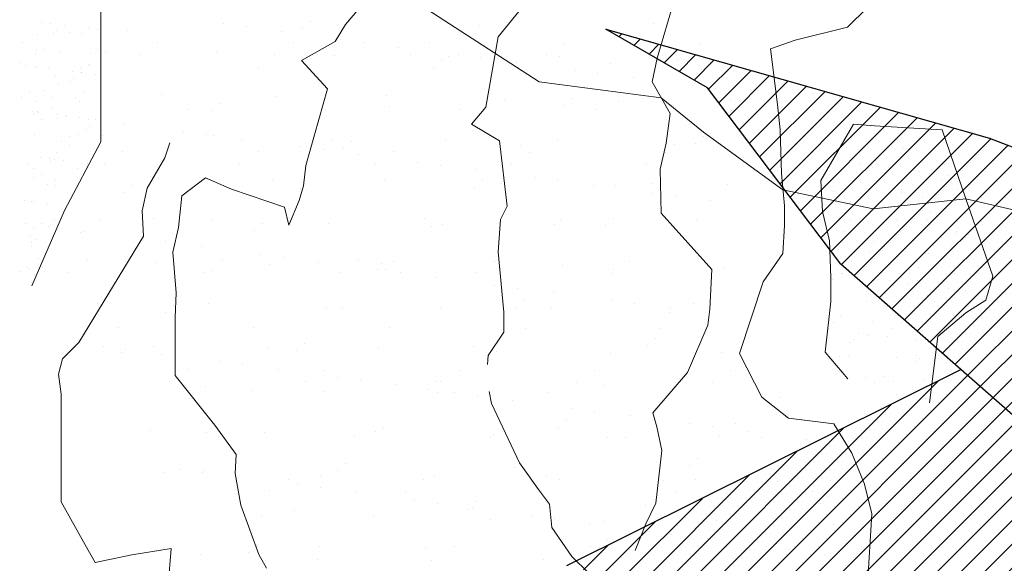
# Model space of a CAD drawing. Units: inches. Extents: x 1986 to 21484, y -1816 to 2016.
# Tile 17 of 85: x 2148.647 to 2157.681, y 1882.437 to 1887.425. Entities that reach past the tile are written whole.
import ezdxf

# ---------------------------------------------------------------- set-up
doc = ezdxf.new("R2010")
doc.units = ezdxf.units.IN
doc.layers.add('L-PLNT', color=84, linetype='Continuous', lineweight=13)
doc.layers.add('vfolhas', color=114, linetype='Continuous', lineweight=5)
doc.layers.add('vfolhas2', color=102, linetype='Continuous')

# ---------------------------------------------------------------- blocks, each defined once
blk = doc.blocks.new('arbusto_PB_verde_grande')
at = {"layer": 'vfolhas'}
h = blk.add_hatch(dxfattribs=at)
h.set_pattern_fill('ANSI31', color=256, scale=0.05, style=0)
h.set_pattern_definition([(45, (-2446.5133113, 50.986076), (-0.004419417382, 0.004419417382), [])])
h.paths.add_polyline_path([(-0.57219, 0.06233), (-0.7153, 0.10298), (-0.67736, 0.08107), (-0.62769, 0.01536), (-0.56347, -0.04095), (-0.26461, -0.0834), (-0.14874, -0.06595), (-0.10151, -0.05877), (-0.20418, -0.0472), (-0.40279, -0.00339)])
h.paths.add_polyline_path([(-0.56347, -0.04095), (-0.58279, -0.02401), (-0.72992, -0.09726), (-0.4334, -0.1679), (-0.41452, -0.15048), (-0.31518, -0.09101), (-0.26461, -0.0834)])
h.paths.add_polyline_path([(-0.2769, -0.47267), (-0.27429, -0.44776), (-0.16328, -0.25376), (0.02625, -0.03934), (-0.21007, -0.20995), (-0.2672, -0.24466), (-0.36485, -0.35697), (-0.42907, -0.46341), (-0.47586, -0.60425), (-0.37946, -0.57603)])
at = {"layer": 'vfolhas2'}
for p, q in [((-0.67736, 0.08107), (-0.7153, 0.10298)), ((-0.7153, 0.10298), (-0.57219, 0.06233)), ((-0.62769, 0.01536), (-0.67736, 0.08107)), ((-0.57219, 0.06233), (-0.40279, -0.00339)), ((-0.56347, -0.04095), (-0.62769, 0.01536)), ((-0.58279, -0.02401), (-0.72992, -0.09726))]:
    blk.add_line(p, q, dxfattribs=at)
blk = doc.blocks.new('PLANT-SHRUB')
for p, q in [((2149.3904, 1887.9573), (2149.3904, 1887.2965)), ((2151.874, 1887.8531), (2153.4137, 1886.8553)), ((2154.6784, 1887.6913), (2154.4964, 1887.0728)), ((2153.0377, 1887.2662), (2153.2939, 1887.5837)), ((2151.636, 1887.381), (2151.7601, 1887.5256)), ((2156.2426, 1887.3561), (2156.4241, 1887.5374)), ((2151.3125, 1887.4075), (2151.3125, 1887.4075)), ((2148.847, 1887.3985), (2148.847, 1887.3985)), ((2148.9303, 1887.3876), (2148.9303, 1887.3876)), ((2148.9856, 1887.3277), (2148.9856, 1887.3277)), ((2149.0602, 1887.3705), (2149.0602, 1887.3705)), ((2149.2774, 1887.3419), (2149.2774, 1887.3419)), ((2149.3606, 1887.3309), (2149.3606, 1887.3309)), ((2149.6396, 1887.3262), (2149.6396, 1887.3262)), ((2150.5172, 1887.3856), (2150.5172, 1887.3856)), ((2150.7253, 1887.3582), (2150.7253, 1887.3582)), ((2151.0502, 1887.3155), (2151.0502, 1887.3155)), ((2151.2389, 1887.34), (2151.2389, 1887.34)), ((2151.543, 1887.226), (2151.636, 1887.381)), ((2152.8617, 1887.3753), (2152.8617, 1887.3753)), ((2154.461, 1887.389), (2154.461, 1887.389)), ((2155.7616, 1887.2382), (2156.2426, 1887.3561)), ((2156.2426, 1887.3561), (2156.2426, 1887.3561)), ((2148.8099, 1887.2924), (2148.8099, 1887.2924)), ((2148.9562, 1887.3007), (2148.9562, 1887.3007)), ((2149.1052, 1887.3099), (2149.1052, 1887.3099)), ((2149.2189, 1887.2943), (2149.2189, 1887.2943)), ((2149.3904, 1887.2965), (2149.3904, 1886.876)), ((2151.2327, 1887.0503), (2151.543, 1887.226)), ((2151.5931, 1887.244), (2151.5931, 1887.244)), ((2152.9249, 1886.6211), (2153.0377, 1887.2662)), ((2155.5347, 1887.1566), (2155.7616, 1887.2382)), ((2148.6687, 1887.2197), (2148.6687, 1887.2197)), ((2148.797, 1887.1549), (2148.797, 1887.1549)), ((2148.8625, 1887.1553), (2148.8625, 1887.1553)), ((2149.016, 1887.1342), (2149.016, 1887.1342)), ((2149.3603, 1887.1543), (2149.3603, 1887.1543)), ((2149.4326, 1887.1303), (2149.4326, 1887.1303)), ((2149.9133, 1887.2174), (2149.9133, 1887.2174)), ((2150.455, 1887.1352), (2150.455, 1887.1352)), ((2151.1579, 1887.2152), (2151.1579, 1887.2152)), ((2151.8011, 1887.2166), (2151.8011, 1887.2166)), ((2152.126, 1887.1738), (2152.126, 1887.1738)), ((2152.4026, 1887.2129), (2152.4026, 1887.2129)), ((2153.6472, 1887.2106), (2153.6472, 1887.2106)), ((2154.8918, 1887.2084), (2154.8918, 1887.2084)), ((2155.5986, 1886.6458), (2155.5347, 1887.1566)), ((2148.7951, 1887.1123), (2148.7951, 1887.1123)), ((2149.2929, 1887.1114), (2149.2929, 1887.1114)), ((2149.7448, 1887.11), (2149.7448, 1887.11)), ((2150.9894, 1887.1078), (2150.9894, 1887.1078)), ((2151.4706, 1886.7919), (2151.2327, 1887.0503)), ((2151.5345, 1887.0963), (2151.5345, 1887.0963)), ((2152.234, 1887.1055), (2152.234, 1887.1055)), ((2152.514, 1887.0567), (2152.514, 1887.0567)), ((2152.5806, 1887.083), (2152.5806, 1887.083)), ((2152.6689, 1887.1023), (2152.6689, 1887.1023)), ((2152.8769, 1887.075), (2152.8769, 1887.075)), ((2153.4787, 1887.1033), (2153.4787, 1887.1033)), ((2153.603, 1887.0879), (2153.603, 1887.0879)), ((2154.4964, 1887.0728), (2154.4509, 1886.8545)), ((2154.6825, 1887.049), (2154.6825, 1887.049)), ((2154.7233, 1887.101), (2154.7233, 1887.101)), ((2148.6579, 1887.0275), (2148.6579, 1887.0275)), ((2148.6997, 1887.004), (2148.6997, 1887.004)), ((2148.7829, 1886.9931), (2148.7829, 1886.9931)), ((2148.7999, 1886.9843), (2148.7999, 1886.9843)), ((2148.9128, 1886.976), (2148.9128, 1886.976)), ((2149.2088, 1886.9863), (2149.2088, 1886.9863)), ((2149.2776, 1887.0146), (2149.2776, 1887.0146)), ((2149.2919, 1887.0076), (2149.2919, 1887.0076)), ((2150.8411, 1886.9754), (2150.8411, 1886.9754)), ((2152.4403, 1886.9892), (2152.4403, 1886.9892)), ((2153.2019, 1887.0322), (2153.2019, 1887.0322)), ((2153.7447, 1886.9607), (2153.7447, 1886.9607)), ((2154.0632, 1887.0245), (2154.0632, 1887.0245)), ((2148.9761, 1886.9095), (2148.9761, 1886.9095)), ((2149.1091, 1886.8601), (2149.1091, 1886.8601)), ((2149.13, 1886.9474), (2149.13, 1886.9474)), ((2149.1385, 1886.8871), (2149.1385, 1886.8871)), ((2149.2132, 1886.9364), (2149.2132, 1886.9364)), ((2149.2182, 1886.9401), (2149.2182, 1886.9401)), ((2149.3432, 1886.9193), (2149.3432, 1886.9193)), ((2149.3904, 1886.876), (2149.3904, 1886.3054)), ((2153.9528, 1886.9333), (2153.9528, 1886.9333)), ((2154.2777, 1886.8905), (2154.2777, 1886.8905)), ((2148.8684, 1886.7739), (2148.8684, 1886.7739)), ((2149.006, 1886.8262), (2149.006, 1886.8262)), ((2151.2728, 1886.0864), (2151.4706, 1886.7919)), ((2153.4137, 1886.8553), (2154.5328, 1886.7089)), ((2154.4509, 1886.8545), (2154.6147, 1886.5634)), ((2154.8205, 1886.8191), (2154.8205, 1886.8191)), ((2155.0286, 1886.7917), (2155.0286, 1886.7917)), ((2148.666, 1886.712), (2148.666, 1886.712)), ((2148.7334, 1886.7549), (2148.7334, 1886.7549)), ((2148.9499, 1886.7143), (2148.9499, 1886.7143)), ((2149.1638, 1886.7111), (2149.1638, 1886.7111)), ((2149.1988, 1886.6782), (2149.1988, 1886.6782)), ((2149.2312, 1886.754), (2149.2312, 1886.754)), ((2149.9479, 1886.735), (2149.9479, 1886.735)), ((2150.994, 1886.7216), (2150.994, 1886.7216)), ((2152.0164, 1886.7265), (2152.0164, 1886.7265)), ((2153.0959, 1886.6876), (2153.0959, 1886.6876)), ((2153.7155, 1886.7059), (2153.7155, 1886.7059)), ((2154.5328, 1886.7089), (2154.9211, 1886.3936)), ((2155.1645, 1886.6792), (2155.1645, 1886.6792)), ((2155.3535, 1886.7489), (2155.3535, 1886.7489)), ((2148.7898, 1886.6763), (2148.7898, 1886.6763)), ((2148.9526, 1886.6054), (2148.9526, 1886.6054)), ((2150.1973, 1886.6031), (2150.1973, 1886.6031)), ((2150.4197, 1886.5893), (2150.4197, 1886.5893)), ((2150.4934, 1886.6568), (2150.4934, 1886.6568)), ((2151.4419, 1886.6009), (2151.4419, 1886.6009)), ((2152.0425, 1886.6247), (2152.0425, 1886.6247)), ((2152.6865, 1886.5986), (2152.6865, 1886.5986)), ((2152.7917, 1886.4675), (2152.9249, 1886.6211)), ((2153.6418, 1886.6384), (2153.6418, 1886.6384)), ((2153.9312, 1886.5963), (2153.9312, 1886.5963)), ((2154.1421, 1886.6743), (2154.1421, 1886.6743)), ((2155.1758, 1886.5941), (2155.1758, 1886.5941)), ((2155.2646, 1886.6737), (2155.2646, 1886.6737)), ((2155.6244, 1886.4136), (2155.5986, 1886.6458)), ((2148.7654, 1886.5814), (2148.7654, 1886.5814)), ((2148.7814, 1886.5599), (2148.7814, 1886.5599)), ((2148.8109, 1886.5869), (2148.8109, 1886.5869)), ((2148.8204, 1886.5756), (2148.8204, 1886.5756)), ((2148.847, 1886.5092), (2148.847, 1886.5092)), ((2148.9826, 1886.5529), (2148.9826, 1886.5529)), ((2148.9959, 1886.5181), (2148.9959, 1886.5181)), ((2149.0658, 1886.5419), (2149.0658, 1886.5419)), ((2149.0729, 1886.541), (2149.0729, 1886.541)), ((2149.1958, 1886.5248), (2149.1958, 1886.5248)), ((2149.281, 1886.5136), (2149.281, 1886.5136)), ((2149.3448, 1886.5083), (2149.3448, 1886.5083)), ((2154.6147, 1886.5634), (2154.5783, 1886.2905)), ((2149.262, 1886.4196), (2149.262, 1886.4196)), ((2149.2914, 1886.4466), (2149.2914, 1886.4466)), ((2149.6059, 1886.4708), (2149.6059, 1886.4708)), ((2152.7917, 1886.4675), (2152.7917, 1886.4675)), ((2153.0479, 1886.3139), (2152.7917, 1886.4675)), ((2155.6373, 1886.0136), (2155.6244, 1886.4136)), ((2156.2958, 1886.4652), (2155.9988, 1885.9491)), ((2156.4895, 1886.4523), (2156.2958, 1886.4652)), ((2157.1093, 1886.4136), (2156.4895, 1886.4523)), ((2157.3288, 1885.7813), (2157.1093, 1886.4136)), ((2148.7797, 1886.3682), (2148.7797, 1886.3682)), ((2149.1021, 1886.3537), (2149.1021, 1886.3537)), ((2149.1887, 1886.3702), (2149.1887, 1886.3702)), ((2149.4074, 1886.3602), (2149.4074, 1886.3602)), ((2150.1488, 1886.3993), (2150.1488, 1886.3993)), ((2150.3568, 1886.3719), (2150.3568, 1886.3719)), ((2150.4298, 1886.3651), (2150.4298, 1886.3651)), ((2150.6817, 1886.3292), (2150.6817, 1886.3292)), ((2151.5093, 1886.3263), (2151.5093, 1886.3263)), ((2153.5779, 1886.3178), (2153.5779, 1886.3178)), ((2154.9169, 1886.3551), (2154.9169, 1886.3551)), ((2154.9211, 1886.3936), (2155.6502, 1885.8652)), ((2156.2786, 1886.3449), (2156.2786, 1886.3449)), ((2156.7369, 1886.3459), (2156.7369, 1886.3459)), ((2156.9009, 1886.3437), (2156.9009, 1886.3437)), ((2149.0347, 1886.3107), (2149.0347, 1886.3107)), ((2149.3904, 1886.3054), (2149.0597, 1885.6747)), ((2149.1029, 1886.2738), (2149.1029, 1886.2738)), ((2150.0259, 1886.2961), (2149.9795, 1886.157)), ((2151.2246, 1886.2577), (2151.2246, 1886.2577)), ((2151.4326, 1886.2303), (2151.4326, 1886.2303)), ((2151.6212, 1886.2385), (2151.6212, 1886.2385)), ((2151.6948, 1886.3061), (2151.6948, 1886.3061)), ((2152.5555, 1886.3129), (2152.5555, 1886.3129)), ((2153.1193, 1885.7143), (2153.0479, 1886.3139)), ((2153.244, 1886.2739), (2153.244, 1886.2739)), ((2154.5783, 1886.2905), (2154.5237, 1886.054)), ((2154.6573, 1886.2789), (2154.6573, 1886.2789)), ((2154.8433, 1886.2876), (2154.8433, 1886.2876)), ((2156.2313, 1886.2553), (2156.2313, 1886.2553)), ((2156.7001, 1886.3122), (2156.7001, 1886.3122)), ((2156.7544, 1886.2486), (2156.7544, 1886.2486)), ((2148.8352, 1886.1583), (2148.8352, 1886.1583)), ((2148.9184, 1886.1474), (2148.9184, 1886.1474)), ((2148.9638, 1886.1463), (2148.9638, 1886.1463)), ((2148.9858, 1886.2101), (2148.9858, 1886.2101)), ((2149.5905, 1886.2166), (2149.5905, 1886.2166)), ((2149.9795, 1886.157), (2149.8169, 1885.8786)), ((2150.0219, 1886.2248), (2150.0219, 1886.2248)), ((2150.8351, 1886.2143), (2150.8351, 1886.2143)), ((2151.7575, 1886.1875), (2151.7575, 1886.1875)), ((2152.0798, 1886.2121), (2152.0798, 1886.2121)), ((2153.3244, 1886.2098), (2153.3244, 1886.2098)), ((2154.569, 1886.2075), (2154.569, 1886.2075)), ((2156.5975, 1886.1505), (2156.5975, 1886.1505)), ((2148.7179, 1886.1089), (2148.7179, 1886.1089)), ((2148.7697, 1886.0602), (2148.7697, 1886.0602)), ((2148.9343, 1886.1193), (2148.9343, 1886.1193)), ((2149.0484, 1886.1303), (2149.0484, 1886.1303)), ((2149.1786, 1886.0622), (2149.1786, 1886.0622)), ((2149.2157, 1886.108), (2149.2157, 1886.108)), ((2149.2655, 1886.1017), (2149.2655, 1886.1017)), ((2149.422, 1886.1092), (2149.422, 1886.1092)), ((2150.6666, 1886.107), (2150.6666, 1886.107)), ((2151.2521, 1885.9004), (2151.2728, 1886.0864)), ((2151.9112, 1886.1047), (2151.9112, 1886.1047)), ((2152.3004, 1886.1161), (2152.3004, 1886.1161)), ((2152.5084, 1886.0887), (2152.5084, 1886.0887)), ((2152.8334, 1886.0459), (2152.8334, 1886.0459)), ((2153.1559, 1886.1024), (2153.1559, 1886.1024)), ((2154.4005, 1886.1002), (2154.4005, 1886.1002)), ((2154.5237, 1886.054), (2154.5332, 1885.65)), ((2156.354, 1886.0998), (2156.354, 1886.0998)), ((2156.4581, 1886.0861), (2156.4581, 1886.0861)), ((2156.4723, 1886.0703), (2156.4723, 1886.0703)), ((2156.5012, 1886.1299), (2156.5012, 1886.1299)), ((2156.5132, 1886.0968), (2156.5132, 1886.0968)), ((2156.6205, 1886.0647), (2156.6205, 1886.0647)), ((2157.0121, 1886.0509), (2157.0121, 1886.0509)), ((2157.1356, 1886.0957), (2157.1356, 1886.0957)), ((2148.7752, 1885.9735), (2148.7752, 1885.9735)), ((2148.8432, 1886.0038), (2148.8432, 1886.0038)), ((2149.9227, 1885.9649), (2149.9227, 1885.9649)), ((2150.1352, 1885.8074), (2150.3524, 1885.9727)), ((2150.3524, 1885.9727), (2150.5903, 1885.8694)), ((2150.3524, 1885.9727), (2150.3524, 1885.9727)), ((2151.9913, 1885.9564), (2151.9913, 1885.9564)), ((2152.8963, 1885.9553), (2152.8963, 1885.9553)), ((2153.3762, 1885.9744), (2153.3762, 1885.9744)), ((2155.6631, 1885.7168), (2155.6373, 1886.0136)), ((2156.3274, 1885.9706), (2156.3274, 1885.9706)), ((2156.892, 1886.029), (2156.892, 1886.029)), ((2156.996, 1886.0153), (2156.996, 1886.0153)), ((2157.1584, 1885.9939), (2157.1584, 1885.9939)), ((2148.9056, 1885.9104), (2148.9056, 1885.9104)), ((2148.973, 1885.9534), (2148.973, 1885.9534)), ((2148.9758, 1885.9021), (2148.9758, 1885.9021)), ((2149.6742, 1885.9062), (2149.6742, 1885.9062)), ((2149.8169, 1885.8786), (2149.7705, 1885.6698)), ((2150.5903, 1885.8694), (2151.0763, 1885.7041)), ((2150.9689, 1885.9515), (2150.9689, 1885.9515)), ((2151.2108, 1885.7661), (2151.2521, 1885.9004)), ((2151.2234, 1885.874), (2151.2234, 1885.874)), ((2152.8226, 1885.8878), (2152.8226, 1885.8878)), ((2153.0707, 1885.9175), (2153.0707, 1885.9175)), ((2153.5843, 1885.947), (2153.5843, 1885.947)), ((2153.9092, 1885.9043), (2153.9092, 1885.9043)), ((2154.1169, 1885.9042), (2154.1169, 1885.9042)), ((2154.4455, 1885.9231), (2154.4455, 1885.9231)), ((2155.1393, 1885.9091), (2155.1393, 1885.9091)), ((2155.6502, 1885.8652), (2156.4772, 1885.6891)), ((2155.9988, 1885.9491), (2156.0118, 1885.6652)), ((2156.2188, 1885.8702), (2156.2188, 1885.8702)), ((2156.2905, 1885.9368), (2156.2905, 1885.9368)), ((2157.1019, 1885.9545), (2157.1019, 1885.9545)), ((2157.253, 1885.866), (2157.253, 1885.866)), ((2149.6005, 1885.8387), (2149.6005, 1885.8387)), ((2150.1042, 1885.518), (2150.1352, 1885.8074)), ((2150.1352, 1885.8074), (2150.1352, 1885.8074)), ((2154.452, 1885.8328), (2154.452, 1885.8328)), ((2154.6601, 1885.8054), (2154.6601, 1885.8054)), ((2156.1172, 1885.8445), (2156.1172, 1885.8445)), ((2156.4772, 1885.6891), (2157.3288, 1885.7813)), ((2156.7395, 1885.8433), (2156.7395, 1885.8433)), ((2156.7418, 1885.8635), (2156.7418, 1885.8635)), ((2156.9281, 1885.7952), (2156.9281, 1885.7952)), ((2157.3288, 1885.7813), (2158.2522, 1885.5676)), ((2157.5742, 1885.0717), (2157.3288, 1885.7813)), ((2148.6878, 1885.7638), (2148.6878, 1885.7638)), ((2148.7596, 1885.7522), (2148.7596, 1885.7522)), ((2148.771, 1885.7529), (2148.771, 1885.7529)), ((2148.901, 1885.7357), (2148.901, 1885.7357)), ((2151.0763, 1885.7041), (2151.1177, 1885.5387)), ((2151.1177, 1885.5387), (2151.2108, 1885.7661)), ((2151.2108, 1885.7661), (2151.2108, 1885.7661)), ((2153.0578, 1885.5914), (2153.1193, 1885.7143)), ((2153.1193, 1885.7143), (2153.1193, 1885.7143)), ((2154.985, 1885.7626), (2154.985, 1885.7626)), ((2155.6631, 1885.5362), (2155.6631, 1885.7168)), ((2156.0916, 1885.7546), (2156.0916, 1885.7546)), ((2156.4597, 1885.6853), (2156.4597, 1885.6853)), ((2156.8913, 1885.7615), (2156.8913, 1885.7615)), ((2149.0597, 1885.6747), (2148.7592, 1884.9839)), ((2148.9657, 1885.594), (2148.9657, 1885.594)), ((2149.7705, 1885.6698), (2149.7821, 1885.4378)), ((2149.8745, 1885.6023), (2149.8745, 1885.6023)), ((2150.4046, 1885.595), (2150.4046, 1885.595)), ((2151.1191, 1885.6001), (2151.1191, 1885.6001)), ((2152.3637, 1885.5978), (2152.3637, 1885.5978)), ((2153.6084, 1885.5955), (2153.6084, 1885.5955)), ((2154.0978, 1885.6045), (2154.0978, 1885.6045)), ((2154.5332, 1885.65), (2154.9975, 1885.1315)), ((2156.0118, 1885.6652), (2156.0763, 1885.3943)), ((2156.1698, 1885.6066), (2156.1698, 1885.6066)), ((2156.3519, 1885.5964), (2156.3519, 1885.5964)), ((2156.4361, 1885.6501), (2156.4361, 1885.6501)), ((2156.9742, 1885.5952), (2156.9742, 1885.5952)), ((2156.9995, 1885.6658), (2156.9995, 1885.6658)), ((2157.0584, 1885.6489), (2157.0584, 1885.6489)), ((2148.7044, 1885.5547), (2148.7044, 1885.5547)), ((2148.7765, 1885.5101), (2148.7765, 1885.5101)), ((2148.8439, 1885.553), (2148.8439, 1885.553)), ((2148.9125, 1885.5273), (2148.9125, 1885.5273)), ((2148.9281, 1885.5329), (2148.9281, 1885.5329)), ((2149.3823, 1885.5901), (2149.3823, 1885.5901)), ((2150.0525, 1885.2907), (2150.1042, 1885.518)), ((2150.1042, 1885.518), (2150.1042, 1885.518)), ((2150.8756, 1885.5554), (2150.8756, 1885.5554)), ((2151.4841, 1885.5562), (2151.4841, 1885.5562)), ((2152.4248, 1885.5232), (2152.4248, 1885.5232)), ((2152.5303, 1885.5428), (2152.5303, 1885.5428)), ((2153.0373, 1885.2944), (2153.0578, 1885.5914)), ((2153.5527, 1885.5477), (2153.5527, 1885.5477)), ((2154.0241, 1885.537), (2154.0241, 1885.537)), ((2154.6322, 1885.5088), (2154.6322, 1885.5088)), ((2154.853, 1885.5933), (2154.853, 1885.5933)), ((2155.6502, 1885.2781), (2155.6631, 1885.5362)), ((2156.2738, 1885.5929), (2156.2738, 1885.5929)), ((2156.4363, 1885.5716), (2156.4363, 1885.5716)), ((2156.6924, 1885.5792), (2156.6924, 1885.5792)), ((2156.7077, 1885.5358), (2156.7077, 1885.5358)), ((2156.8117, 1885.5221), (2156.8117, 1885.5221)), ((2148.7495, 1885.4441), (2148.7495, 1885.4441)), ((2149.7821, 1885.4378), (2149.1901, 1884.4635)), ((2149.2027, 1885.4742), (2149.2027, 1885.4742)), ((2149.2374, 1885.4845), (2149.2374, 1885.4845)), ((2150.802, 1885.4879), (2150.802, 1885.4879)), ((2156.2062, 1885.4852), (2156.2062, 1885.4852)), ((2156.5185, 1885.4199), (2156.5185, 1885.4199)), ((2156.7293, 1885.4785), (2156.7293, 1885.4785)), ((2156.9742, 1885.5007), (2156.9742, 1885.5007)), ((2157.2405, 1885.4809), (2157.2405, 1885.4809)), ((2157.2456, 1885.465), (2157.2456, 1885.465)), ((2157.3496, 1885.4513), (2157.3496, 1885.4513)), ((2148.7536, 1885.3412), (2148.7536, 1885.3412)), ((2148.7596, 1885.3785), (2148.7596, 1885.3785)), ((2148.789, 1885.4055), (2148.789, 1885.4055)), ((2149.7803, 1885.413), (2149.7803, 1885.413)), ((2149.9883, 1885.3856), (2149.9883, 1885.3856)), ((2150.3132, 1885.3429), (2150.3132, 1885.3429)), ((2156.0763, 1885.3943), (2156.0892, 1885.0588)), ((2156.4817, 1885.3861), (2156.4817, 1885.3861)), ((2156.5781, 1885.3429), (2156.5781, 1885.3429)), ((2157.2004, 1885.3418), (2157.2004, 1885.3418)), ((2157.2931, 1885.4038), (2157.2931, 1885.4038)), ((2148.818, 1885.2337), (2148.818, 1885.2337)), ((2150.0835, 1884.9187), (2150.0525, 1885.2907)), ((2150.8561, 1885.2714), (2150.8561, 1885.2714)), ((2151.0641, 1885.244), (2151.0641, 1885.244)), ((2153.0885, 1884.7414), (2153.0373, 1885.2944)), ((2155.4694, 1885.0201), (2155.6502, 1885.2781)), ((2156.4472, 1885.3002), (2156.4472, 1885.3002)), ((2156.9869, 1885.2808), (2156.9869, 1885.2808)), ((2157.1192, 1885.2445), (2157.1192, 1885.2445)), ((2148.7148, 1885.1527), (2148.7148, 1885.1527)), ((2148.855, 1885.1556), (2148.855, 1885.1556)), ((2149.2677, 1885.2158), (2149.2677, 1885.2158)), ((2149.8975, 1885.1948), (2149.8975, 1885.1948)), ((2150.5124, 1885.2135), (2150.5124, 1885.2135)), ((2150.9437, 1885.1814), (2150.9437, 1885.1814)), ((2151.389, 1885.2012), (2151.389, 1885.2012)), ((2151.757, 1885.2113), (2151.757, 1885.2113)), ((2151.9661, 1885.1863), (2151.9661, 1885.1863)), ((2152.0771, 1885.2046), (2152.0771, 1885.2046)), ((2153.0016, 1885.209), (2153.0016, 1885.209)), ((2153.0455, 1885.1474), (2153.0455, 1885.1474)), ((2153.6263, 1885.1725), (2153.6263, 1885.1725)), ((2154.2463, 1885.2067), (2154.2463, 1885.2067)), ((2156.2747, 1885.1497), (2156.2747, 1885.1497)), ((2156.2828, 1885.2039), (2156.2828, 1885.2039)), ((2156.8971, 1885.1485), (2156.8971, 1885.1485)), ((2157.0824, 1885.2107), (2157.0824, 1885.2107)), ((2157.5194, 1885.1474), (2157.5194, 1885.1474)), ((2148.6474, 1885.1098), (2148.6474, 1885.1098)), ((2148.7394, 1885.1361), (2148.7394, 1885.1361)), ((2148.7813, 1885.0881), (2148.7813, 1885.0881)), ((2149.0992, 1885.1084), (2149.0992, 1885.1084)), ((2150.3438, 1885.1061), (2150.3438, 1885.1061)), ((2150.4042, 1885.1234), (2150.4042, 1885.1234)), ((2151.5885, 1885.1039), (2151.5885, 1885.1039)), ((2151.9319, 1885.1298), (2151.9319, 1885.1298)), ((2152.0034, 1885.1371), (2152.0034, 1885.1371)), ((2152.1399, 1885.1024), (2152.1399, 1885.1024)), ((2152.4649, 1885.0596), (2152.4649, 1885.0596)), ((2152.8331, 1885.1016), (2152.8331, 1885.1016)), ((2154.0777, 1885.0994), (2154.0777, 1885.0994)), ((2154.0917, 1885.1341), (2154.0917, 1885.1341)), ((2154.9975, 1885.1315), (2154.9792, 1884.7677)), ((2155.1141, 1885.139), (2155.1141, 1885.139)), ((2156.0892, 1885.0588), (2156.0892, 1884.8394)), ((2156.0896, 1885.0998), (2156.0896, 1885.0998)), ((2156.1905, 1885.096), (2156.1905, 1885.096)), ((2156.1936, 1885.1001), (2156.1936, 1885.1001)), ((2156.252, 1885.0784), (2156.252, 1885.0784)), ((2156.7167, 1885.0934), (2156.7167, 1885.0934)), ((2156.8128, 1885.0948), (2156.8128, 1885.0948)), ((2157.2279, 1885.0959), (2157.2279, 1885.0959)), ((2157.4351, 1885.0937), (2157.4351, 1885.0937)), ((2157.5096, 1884.8524), (2157.5742, 1885.0717)), ((2148.7592, 1884.9839), (2148.7592, 1884.9839)), ((2153.0077, 1884.9881), (2153.0077, 1884.9881)), ((2155.2499, 1884.3621), (2155.4694, 1885.0201)), ((2156.1089, 1885.0446), (2156.1089, 1885.0446)), ((2156.5235, 1885.0427), (2156.5235, 1885.0427)), ((2156.6275, 1885.029), (2156.6275, 1885.029)), ((2156.7899, 1885.0076), (2156.7899, 1885.0076)), ((2156.8835, 1885.0285), (2156.8835, 1885.0285)), ((2157.0614, 1884.9719), (2157.0614, 1884.9719)), ((2150.075, 1884.6914), (2150.0835, 1884.9187)), ((2153.2158, 1884.9607), (2153.2158, 1884.9607)), ((2153.5407, 1884.918), (2153.5407, 1884.918)), ((2156.4346, 1884.9152), (2156.4346, 1884.9152)), ((2156.9743, 1884.8958), (2156.9743, 1884.8958)), ((2157.1654, 1884.9582), (2157.1654, 1884.9582)), ((2157.3279, 1884.9368), (2157.3279, 1884.9368)), ((2157.4974, 1884.8891), (2157.4974, 1884.8891)), ((2149.3571, 1884.82), (2149.3571, 1884.82)), ((2150.0565, 1884.8048), (2150.0565, 1884.8048)), ((2150.3795, 1884.825), (2150.3795, 1884.825)), ((2151.4589, 1884.7861), (2151.4589, 1884.7861)), ((2153.2049, 1884.7863), (2153.2049, 1884.7863)), ((2153.2786, 1884.8538), (2153.2786, 1884.8538)), ((2154.0836, 1884.8465), (2154.0836, 1884.8465)), ((2154.2916, 1884.8191), (2154.2916, 1884.8191)), ((2154.8277, 1884.8217), (2154.8277, 1884.8217)), ((2156.0892, 1884.8394), (2156.0376, 1884.375)), ((2156.4167, 1884.8425), (2156.4167, 1884.8425)), ((2156.6728, 1884.8354), (2156.6728, 1884.8354)), ((2156.7096, 1884.8692), (2156.7096, 1884.8692)), ((2157.039, 1884.8414), (2157.039, 1884.8414)), ((2157.3288, 1884.7362), (2157.5096, 1884.8524)), ((2157.4842, 1884.8531), (2157.4842, 1884.8531)), ((2149.9828, 1884.7373), (2149.9828, 1884.7373)), ((2150.075, 1884.1595), (2150.075, 1884.6914)), ((2151.6056, 1884.7726), (2151.6056, 1884.7726)), ((2152.5051, 1884.7727), (2152.5051, 1884.7727)), ((2153.0885, 1884.7414), (2153.0885, 1884.7414)), ((2153.0885, 1884.5571), (2153.0885, 1884.7414)), ((2153.5275, 1884.7776), (2153.5275, 1884.7776)), ((2154.607, 1884.7387), (2154.607, 1884.7387)), ((2154.6165, 1884.7763), (2154.6165, 1884.7763)), ((2154.9792, 1884.7677), (2154.961, 1884.6222)), ((2156.181, 1884.7151), (2156.181, 1884.7151)), ((2156.7041, 1884.7084), (2156.7041, 1884.7084)), ((2157.0706, 1884.5169), (2157.3288, 1884.7362)), ((2157.2153, 1884.7108), (2157.2153, 1884.7108)), ((2149.5517, 1884.6015), (2149.5517, 1884.6015)), ((2154.961, 1884.6222), (2154.775, 1884.1886)), ((2154.961, 1884.6222), (2154.961, 1884.6222)), ((2156.1133, 1884.6492), (2156.1133, 1884.6492)), ((2156.4739, 1884.6532), (2156.4739, 1884.6532)), ((2156.7357, 1884.6481), (2156.7357, 1884.6481)), ((2150.7963, 1884.5992), (2150.7963, 1884.5992)), ((2152.0409, 1884.597), (2152.0409, 1884.597)), ((2152.945, 1884.3421), (2153.0885, 1884.5571)), ((2153.2856, 1884.5947), (2153.2856, 1884.5947)), ((2154.5302, 1884.5925), (2154.5302, 1884.5925)), ((2156.0678, 1884.5853), (2156.0678, 1884.5853)), ((2156.3392, 1884.5495), (2156.3392, 1884.5495)), ((2156.422, 1884.5302), (2156.422, 1884.5302)), ((2156.4432, 1884.5358), (2156.4432, 1884.5358)), ((2156.6057, 1884.5144), (2156.6057, 1884.5144)), ((2156.6514, 1884.5944), (2156.6514, 1884.5944)), ((2156.9617, 1884.5107), (2156.9617, 1884.5107)), ((2156.9931, 1883.9105), (2157.0706, 1884.5169)), ((2149.1901, 1884.4635), (2149.0392, 1884.3127)), ((2149.4118, 1884.4267), (2149.4118, 1884.4267)), ((2149.8723, 1884.4247), (2149.8723, 1884.4247)), ((2151.2579, 1884.454), (2151.2579, 1884.454)), ((2152.8071, 1884.4218), (2152.8071, 1884.4218)), ((2154.4064, 1884.4356), (2154.4064, 1884.4356)), ((2154.48, 1884.5031), (2154.48, 1884.5031)), ((2156.2632, 1884.4601), (2156.2632, 1884.4601)), ((2156.3001, 1884.4939), (2156.3001, 1884.4939)), ((2156.8771, 1884.4787), (2156.8771, 1884.4787)), ((2156.9811, 1884.465), (2156.9811, 1884.465)), ((2149.585, 1884.3728), (2149.585, 1884.3728)), ((2149.6198, 1884.3993), (2149.6198, 1884.3993)), ((2149.9447, 1884.3566), (2149.9447, 1884.3566)), ((2150.9185, 1884.4113), (2150.9185, 1884.4113)), ((2151.1843, 1884.3865), (2151.1843, 1884.3865)), ((2151.9409, 1884.4162), (2151.9409, 1884.4162)), ((2152.9398, 1884.2617), (2152.945, 1884.3421)), ((2152.945, 1884.3421), (2152.945, 1884.3421)), ((2153.0204, 1884.3773), (2153.0204, 1884.3773)), ((2154.0665, 1884.364), (2154.0665, 1884.364)), ((2155.0889, 1884.3689), (2155.0889, 1884.3689)), ((2155.2499, 1884.3621), (2155.2499, 1884.3621)), ((2155.4565, 1883.9621), (2155.2499, 1884.3621)), ((2156.0376, 1884.375), (2156.2442, 1884.1298)), ((2156.1684, 1884.33), (2156.1684, 1884.33)), ((2156.2553, 1884.3421), (2156.2553, 1884.3421)), ((2156.8776, 1884.341), (2156.8776, 1884.341)), ((2149.0392, 1884.3127), (2149.0044, 1884.1735)), ((2150.4876, 1884.2851), (2150.4876, 1884.2851)), ((2150.6956, 1884.2577), (2150.6956, 1884.2577)), ((2156.6915, 1884.3233), (2156.6915, 1884.3233)), ((2156.864, 1884.2847), (2156.864, 1884.2847)), ((2156.9008, 1884.3185), (2156.9008, 1884.3185)), ((2149.0044, 1884.1735), (2149.0276, 1883.9879)), ((2150.4369, 1883.7048), (2150.075, 1884.1595)), ((2150.1896, 1884.2127), (2150.1896, 1884.2127)), ((2151.0205, 1884.2149), (2151.0205, 1884.2149)), ((2151.4342, 1884.2104), (2151.4342, 1884.2104)), ((2152.6788, 1884.2082), (2152.6788, 1884.2082)), ((2153.9235, 1884.2059), (2153.9235, 1884.2059)), ((2154.775, 1884.1886), (2154.4569, 1883.8163)), ((2155.1681, 1884.2037), (2155.1681, 1884.2037)), ((2150.021, 1884.1053), (2150.021, 1884.1053)), ((2151.2657, 1884.1031), (2151.2657, 1884.1031)), ((2151.5634, 1884.1435), (2151.5634, 1884.1435)), ((2151.7714, 1884.1161), (2151.7714, 1884.1161)), ((2152.0964, 1884.0733), (2152.0964, 1884.0733)), ((2152.4594, 1884.1032), (2152.4594, 1884.1032)), ((2152.5103, 1884.1008), (2152.5103, 1884.1008)), ((2153.7549, 1884.0985), (2153.7549, 1884.0985)), ((2154.0086, 1884.071), (2154.0086, 1884.071)), ((2154.9996, 1884.0963), (2154.9996, 1884.0963)), ((2156.4094, 1884.1451), (2156.4094, 1884.1451)), ((2156.49, 1884.094), (2156.49, 1884.094)), ((2156.5743, 1884.1477), (2156.5743, 1884.1477)), ((2156.665, 1884.1025), (2156.665, 1884.1025)), ((2156.9491, 1884.1257), (2156.9491, 1884.1257)), ((2149.0276, 1883.9879), (2149.0276, 1883.002)), ((2150.3543, 1884.0549), (2150.3543, 1884.0549)), ((2150.7865, 1884.022), (2150.7865, 1884.022)), ((2151.4338, 1884.016), (2151.4338, 1884.016)), ((2152.3857, 1884.0357), (2152.3857, 1884.0357)), ((2152.4799, 1884.0026), (2152.4799, 1884.0026)), ((2152.6392, 1884.0018), (2152.6392, 1884.0018)), ((2152.8473, 1883.9744), (2152.8473, 1883.9744)), ((2152.9758, 1883.9017), (2152.9553, 1884.0144)), ((2153.5023, 1884.0075), (2153.5023, 1884.0075)), ((2154.5818, 1883.9686), (2154.5818, 1883.9686)), ((2156.6929, 1883.9856), (2156.6929, 1883.9856)), ((2156.7969, 1883.9719), (2156.7969, 1883.9719)), ((2153.232, 1883.359), (2152.9758, 1883.9017)), ((2153.1722, 1883.9317), (2153.1722, 1883.9317)), ((2155.7019, 1883.7685), (2155.4565, 1883.9621)), ((2155.628, 1883.9553), (2155.628, 1883.9553)), ((2156.9594, 1883.9505), (2156.9594, 1883.9505)), ((2153.7151, 1883.8602), (2153.7151, 1883.8602)), ((2153.9231, 1883.8328), (2153.9231, 1883.8328)), ((2154.248, 1883.79), (2154.248, 1883.79)), ((2154.4569, 1883.8163), (2154.4932, 1883.6891)), ((2150.4369, 1883.7048), (2150.4369, 1883.7048)), ((2150.6334, 1883.4361), (2150.4369, 1883.7048)), ((2150.4388, 1883.7034), (2150.4388, 1883.7034)), ((2153.6609, 1883.7524), (2153.6609, 1883.7524)), ((2154.7909, 1883.7186), (2154.7909, 1883.7186)), ((2155.21, 1883.7203), (2155.21, 1883.7203)), ((2155.7019, 1883.7685), (2155.7019, 1883.7685)), ((2156.1151, 1883.7169), (2155.7019, 1883.7685)), ((2156.2829, 1883.446), (2156.1151, 1883.7169)), ((2149.8472, 1883.6546), (2149.8472, 1883.6546)), ((2150.3651, 1883.6359), (2150.3651, 1883.6359)), ((2150.8933, 1883.6412), (2150.8933, 1883.6412)), ((2151.9157, 1883.6461), (2151.9157, 1883.6461)), ((2151.9879, 1883.6712), (2151.9879, 1883.6712)), ((2152.9952, 1883.6073), (2152.9952, 1883.6073)), ((2153.5872, 1883.6849), (2153.5872, 1883.6849)), ((2154.4932, 1883.6891), (2154.5387, 1883.4712)), ((2154.9989, 1883.6912), (2154.9989, 1883.6912)), ((2155.3238, 1883.6484), (2155.3238, 1883.6484)), ((2150.4735, 1883.5984), (2150.4735, 1883.5984)), ((2151.7182, 1883.5962), (2151.7182, 1883.5962)), ((2152.9628, 1883.5939), (2152.9628, 1883.5939)), ((2154.0414, 1883.5939), (2154.0414, 1883.5939)), ((2154.2074, 1883.5916), (2154.2074, 1883.5916)), ((2155.0638, 1883.5988), (2155.0638, 1883.5988)), ((2155.4521, 1883.5894), (2155.4521, 1883.5894)), ((2155.8667, 1883.5769), (2155.8667, 1883.5769)), ((2150.6231, 1883.2605), (2150.6334, 1883.4361)), ((2150.6334, 1883.4361), (2150.6334, 1883.4361)), ((2154.5387, 1883.4712), (2154.4841, 1882.9898)), ((2156.2829, 1883.446), (2156.2829, 1883.446)), ((2156.3991, 1883.1621), (2156.2829, 1883.446)), ((2151.6402, 1883.3526), (2151.6402, 1883.3526)), ((2153.232, 1883.359), (2153.232, 1883.359)), ((2153.4062, 1883.1132), (2153.232, 1883.359)), ((2154.8623, 1883.4016), (2154.8623, 1883.4016)), ((2149.9673, 1883.2713), (2149.9673, 1883.2713)), ((2150.1191, 1883.2988), (2150.1191, 1883.2988)), ((2150.3271, 1883.2714), (2150.3271, 1883.2714)), ((2150.3291, 1883.2848), (2150.3291, 1883.2848)), ((2150.6748, 1882.9711), (2150.6231, 1883.2605)), ((2151.4086, 1883.2459), (2151.4086, 1883.2459)), ((2151.5666, 1883.2851), (2151.5666, 1883.2851)), ((2153.1894, 1883.3204), (2153.1894, 1883.3204)), ((2154.7887, 1883.3341), (2154.7887, 1883.3341)), ((2150.652, 1883.2286), (2150.652, 1883.2286)), ((2151.1114, 1883.2096), (2151.1114, 1883.2096)), ((2151.1949, 1883.1572), (2151.1949, 1883.1572)), ((2152.3561, 1883.2074), (2152.3561, 1883.2074)), ((2152.4548, 1883.2325), (2152.4548, 1883.2325)), ((2153.4772, 1883.2374), (2153.4772, 1883.2374)), ((2153.6007, 1883.2051), (2153.6007, 1883.2051)), ((2154.5566, 1883.1985), (2154.5566, 1883.1985)), ((2154.8453, 1883.2028), (2154.8453, 1883.2028)), ((2155.6028, 1883.1852), (2155.6028, 1883.1852)), ((2156.09, 1883.2006), (2156.09, 1883.2006)), ((2156.4637, 1882.8912), (2156.3991, 1883.1621)), ((2150.9429, 1883.1023), (2150.9429, 1883.1023)), ((2151.4029, 1883.1298), (2151.4029, 1883.1298)), ((2151.7279, 1883.087), (2151.7279, 1883.087)), ((2152.1875, 1883.1), (2152.1875, 1883.1)), ((2153.4062, 1883.1132), (2153.4062, 1883.1132)), ((2153.5087, 1882.9801), (2153.4062, 1883.1132)), ((2153.4321, 1883.0977), (2153.4321, 1883.0977)), ((2154.6768, 1883.0955), (2154.6768, 1883.0955)), ((2155.9214, 1883.0932), (2155.9214, 1883.0932)), ((2149.0276, 1883.002), (2149.2481, 1882.6076)), ((2152.2707, 1883.0155), (2152.2707, 1883.0155)), ((2152.4788, 1882.9881), (2152.4788, 1882.9881)), ((2152.8417, 1883.0018), (2152.8417, 1883.0018)), ((2153.5292, 1882.765), (2153.5087, 1882.9801)), ((2154.4841, 1882.9898), (2154.3932, 1882.7991)), ((2155.9901, 1882.9834), (2155.9901, 1882.9834)), ((2156.0638, 1883.0509), (2156.0638, 1883.0509)), ((2150.8403, 1882.5164), (2150.6748, 1882.9711)), ((2151.1687, 1882.9206), (2151.1687, 1882.9206)), ((2152.768, 1882.9343), (2152.768, 1882.9343)), ((2152.8037, 1882.9454), (2152.8037, 1882.9454)), ((2154.3909, 1882.9696), (2154.3909, 1882.9696)), ((2156.412, 1882.0396), (2156.4637, 1882.8912)), ((2150.8682, 1882.8711), (2150.8682, 1882.8711)), ((2151.8905, 1882.876), (2151.8905, 1882.876)), ((2152.97, 1882.8372), (2152.97, 1882.8372)), ((2153.3466, 1882.8739), (2153.3466, 1882.8739)), ((2153.5546, 1882.8465), (2153.5546, 1882.8465)), ((2153.8795, 1882.8037), (2153.8795, 1882.8037)), ((2154.0162, 1882.8238), (2154.0162, 1882.8238)), ((2154.3932, 1882.7991), (2154.2933, 1882.5539)), ((2155.0386, 1882.8287), (2155.0386, 1882.8287)), ((2153.7137, 1882.4988), (2153.5292, 1882.765)), ((2154.4224, 1882.7323), (2154.4224, 1882.7323)), ((2154.6304, 1882.7049), (2154.6304, 1882.7049)), ((2156.1181, 1882.7898), (2156.1181, 1882.7898)), ((2154.0431, 1882.651), (2154.0431, 1882.651)), ((2154.9553, 1882.6621), (2154.9553, 1882.6621)), ((2155.5923, 1882.6188), (2155.5923, 1882.6188)), ((2149.2481, 1882.6076), (2149.341, 1882.4452)), ((2149.6776, 1882.5148), (2150.0375, 1882.5728)), ((2150.0375, 1882.5728), (2149.9922, 1881.9992)), ((2150.7474, 1882.5344), (2150.7474, 1882.5344)), ((2150.821, 1882.6019), (2150.821, 1882.6019)), ((2151.3954, 1882.5953), (2151.3954, 1882.5953)), ((2152.3702, 1882.5698), (2152.3702, 1882.5698)), ((2152.64, 1882.5931), (2152.64, 1882.5931)), ((2153.8846, 1882.5908), (2153.8846, 1882.5908)), ((2153.9695, 1882.5835), (2153.9695, 1882.5835)), ((2155.1293, 1882.5886), (2155.1293, 1882.5886)), ((2155.4982, 1882.5906), (2155.4982, 1882.5906)), ((2155.7062, 1882.5632), (2155.7062, 1882.5632)), ((2156.3739, 1882.5863), (2156.3739, 1882.5863)), ((2149.341, 1882.4452), (2149.6776, 1882.5148)), ((2149.341, 1882.4452), (2149.341, 1882.4452)), ((2150.3039, 1882.5147), (2150.3039, 1882.5147)), ((2150.9127, 1882.3924), (2150.8403, 1882.5164)), ((2151.3834, 1882.4758), (2151.3834, 1882.4758)), ((2152.4296, 1882.4624), (2152.4296, 1882.4624)), ((2153.452, 1882.4673), (2153.452, 1882.4673)), ((2153.8674, 1882.3451), (2153.7137, 1882.4988)), ((2156.0312, 1882.5205), (2156.0312, 1882.5205))]:
    blk.add_line(p, q)

msp = doc.modelspace()

# ---------------------------------------------------------------- block references
at = {"layer": 'L-PLNT'}
msp.add_blockref('PLANT-SHRUB', (0, 0), dxfattribs=at)
at = {"layer": 'L-PLNT', "xscale": 24.60366729364114, "yscale": 24.60366729364114, "zscale": 24.60366729364114}
msp.add_blockref('arbusto_PB_verde_grande', (2171.6234, 1884.8051), dxfattribs=at)

doc.saveas('drawing.dxf')
